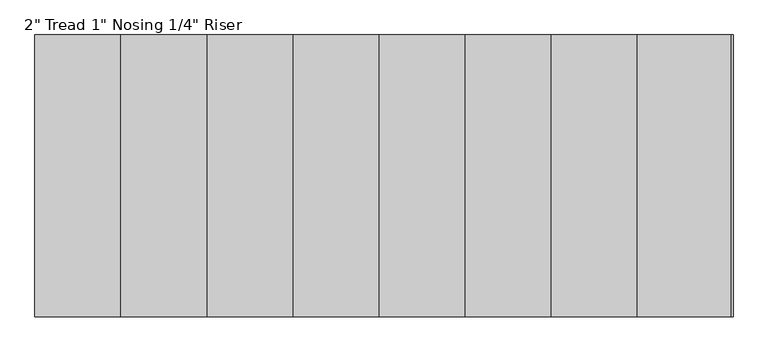
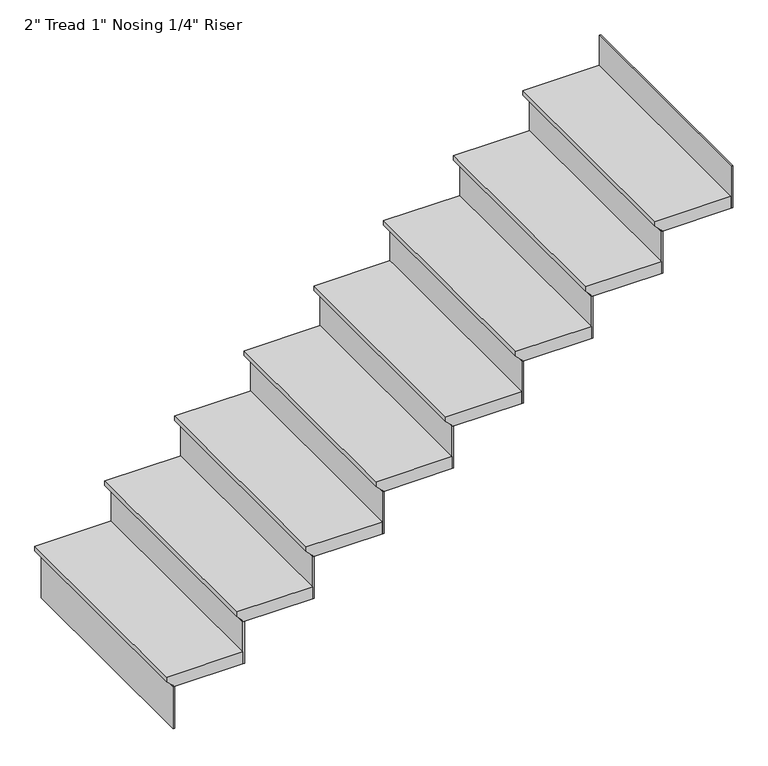
"""IFC4 building model written with IfcOpenShell, lengths in millimetres: stair flight geometry."""

from ifc_helpers import new_model, si_unit, frame, origin, place, context, project, spatial, polyline, outline, extrude, source, transform, mapped, element, save


def stair_flight_0914375a(model_context):
    return source(origin(), model_context, "Body", "SweptSolid", [
        extrude(outline(polyline([(1778.0, -5177.7681702), (1778.0, -5482.5681702), (1758.95, -5482.5681702), (1733.55, -5457.1681702), (1727.2, -5457.1681702), (1727.2, -5177.7681702), (1778.0, -5177.7681702)])), frame((0.0, -6800.457676, 0.0), z_axis=(0.0, 1.0, 0.0), x_axis=(0.0, 0.0, 1.0)), (0.0, 0.0, 1.0), 914.4),
        extrude(outline(polyline([(-5450.8181702, -6800.457676), (-5457.1681702, -6800.457676), (-5457.1681702, -5886.057676), (-5450.8181702, -5886.057676), (-5450.8181702, -6800.457676)])), frame((0.0, 0.0, 1549.4), z_axis=(0.0, 0.0, 1.0), x_axis=(1.0, 0.0, 0.0)), (0.0, 0.0, 1.0), 177.8),
        extrude(outline(polyline([(-3215.6181702, -6800.457676), (-3221.9681702, -6800.457676), (-3221.9681702, -5886.057676), (-3215.6181702, -5886.057676), (-3215.6181702, -6800.457676)])), frame((0.0, 0.0, 2971.8), z_axis=(0.0, 0.0, 1.0), x_axis=(1.0, 0.0, 0.0)), (0.0, 0.0, 1.0), 177.8),
        extrude(outline(polyline([(-5171.4181702, -6800.457676), (-5177.7681702, -6800.457676), (-5177.7681702, -5886.057676), (-5171.4181702, -5886.057676), (-5171.4181702, -6800.457676)])), frame((0.0, 0.0, 1727.2), z_axis=(0.0, 0.0, 1.0), x_axis=(1.0, 0.0, 0.0)), (0.0, 0.0, 1.0), 177.8),
        extrude(outline(polyline([(1955.8, -4898.3681702), (1955.8, -5203.1681702), (1936.75, -5203.1681702), (1911.35, -5177.7681702), (1905.0, -5177.7681702), (1905.0, -4898.3681702), (1955.8, -4898.3681702)])), frame((0.0, -6800.457676, 0.0), z_axis=(0.0, 1.0, 0.0), x_axis=(0.0, 0.0, 1.0)), (0.0, 0.0, 1.0), 914.4),
        extrude(outline(polyline([(-4892.0181702, -6800.457676), (-4898.3681702, -6800.457676), (-4898.3681702, -5886.057676), (-4892.0181702, -5886.057676), (-4892.0181702, -6800.457676)])), frame((0.0, 0.0, 1905.0), z_axis=(0.0, 0.0, 1.0), x_axis=(1.0, 0.0, 0.0)), (0.0, 0.0, 1.0), 177.8),
        extrude(outline(polyline([(2133.6, -4618.9681702), (2133.6, -4923.7681702), (2114.55, -4923.7681702), (2089.15, -4898.3681702), (2082.8, -4898.3681702), (2082.8, -4618.9681702), (2133.6, -4618.9681702)])), frame((0.0, -6800.457676, 0.0), z_axis=(0.0, 1.0, 0.0), x_axis=(0.0, 0.0, 1.0)), (0.0, 0.0, 1.0), 914.4),
        extrude(outline(polyline([(-4612.6181702, -6800.457676), (-4618.9681702, -6800.457676), (-4618.9681702, -5886.057676), (-4612.6181702, -5886.057676), (-4612.6181702, -6800.457676)])), frame((0.0, 0.0, 2082.8), z_axis=(0.0, 0.0, 1.0), x_axis=(1.0, 0.0, 0.0)), (0.0, 0.0, 1.0), 177.8),
        extrude(outline(polyline([(2311.4, -4339.5681702), (2311.4, -4644.3681702), (2292.35, -4644.3681702), (2266.95, -4618.9681702), (2260.6, -4618.9681702), (2260.6, -4339.5681702), (2311.4, -4339.5681702)])), frame((0.0, -6800.457676, 0.0), z_axis=(0.0, 1.0, 0.0), x_axis=(0.0, 0.0, 1.0)), (0.0, 0.0, 1.0), 914.4),
        extrude(outline(polyline([(-4333.2181702, -6800.457676), (-4339.5681702, -6800.457676), (-4339.5681702, -5886.057676), (-4333.2181702, -5886.057676), (-4333.2181702, -6800.457676)])), frame((0.0, 0.0, 2260.6), z_axis=(0.0, 0.0, 1.0), x_axis=(1.0, 0.0, 0.0)), (0.0, 0.0, 1.0), 177.8),
        extrude(outline(polyline([(2489.2, -4060.1681702), (2489.2, -4364.9681702), (2470.15, -4364.9681702), (2444.75, -4339.5681702), (2438.4, -4339.5681702), (2438.4, -4060.1681702), (2489.2, -4060.1681702)])), frame((0.0, -6800.457676, 0.0), z_axis=(0.0, 1.0, 0.0), x_axis=(0.0, 0.0, 1.0)), (0.0, 0.0, 1.0), 914.4),
        extrude(outline(polyline([(-4053.8181702, -6800.457676), (-4060.1681702, -6800.457676), (-4060.1681702, -5886.057676), (-4053.8181702, -5886.057676), (-4053.8181702, -6800.457676)])), frame((0.0, 0.0, 2438.4), z_axis=(0.0, 0.0, 1.0), x_axis=(1.0, 0.0, 0.0)), (0.0, 0.0, 1.0), 177.8),
        extrude(outline(polyline([(2667.0, -3780.7681702), (2667.0, -4085.5681702), (2647.95, -4085.5681702), (2622.55, -4060.1681702), (2616.2, -4060.1681702), (2616.2, -3780.7681702), (2667.0, -3780.7681702)])), frame((0.0, -6800.457676, 0.0), z_axis=(0.0, 1.0, 0.0), x_axis=(0.0, 0.0, 1.0)), (0.0, 0.0, 1.0), 914.4),
        extrude(outline(polyline([(-3774.4181702, -6800.457676), (-3780.7681702, -6800.457676), (-3780.7681702, -5886.057676), (-3774.4181702, -5886.057676), (-3774.4181702, -6800.457676)])), frame((0.0, 0.0, 2616.2), z_axis=(0.0, 0.0, 1.0), x_axis=(1.0, 0.0, 0.0)), (0.0, 0.0, 1.0), 177.8),
        extrude(outline(polyline([(2844.8, -3501.3681702), (2844.8, -3806.1681702), (2825.75, -3806.1681702), (2800.35, -3780.7681702), (2794.0, -3780.7681702), (2794.0, -3501.3681702), (2844.8, -3501.3681702)])), frame((0.0, -6800.457676, 0.0), z_axis=(0.0, 1.0, 0.0), x_axis=(0.0, 0.0, 1.0)), (0.0, 0.0, 1.0), 914.4),
        extrude(outline(polyline([(-3495.0181702, -6800.457676), (-3501.3681702, -6800.457676), (-3501.3681702, -5886.057676), (-3495.0181702, -5886.057676), (-3495.0181702, -6800.457676)])), frame((0.0, 0.0, 2794.0), z_axis=(0.0, 0.0, 1.0), x_axis=(1.0, 0.0, 0.0)), (0.0, 0.0, 1.0), 177.8),
        extrude(outline(polyline([(3022.6, -3221.9681702), (3022.6, -3526.7681702), (3003.55, -3526.7681702), (2978.15, -3501.3681702), (2971.8, -3501.3681702), (2971.8, -3221.9681702), (3022.6, -3221.9681702)])), frame((0.0, -6800.457676, 0.0), z_axis=(0.0, 1.0, 0.0), x_axis=(0.0, 0.0, 1.0)), (0.0, 0.0, 1.0), 914.4),
    ])


if __name__ == "__main__":
    model = new_model("IFC4")
    model_context = context("Model", 3, world=origin())
    ifc_project = project(units=[si_unit("LENGTHUNIT", "METRE", prefix="MILLI")], contexts=[model_context])
    site = spatial("IfcSite", under=ifc_project)
    building = spatial("IfcBuilding", under=site)
    placement = place(None, origin())
    stair_flight_shape = stair_flight_0914375a(model_context)
    element("IfcStairFlight", 1, ObjectType="2\" Tread 1\" Nosing 1/4\" Riser", at=placement, inside=building, context=model_context, shape_type="MappedRepresentation", body=[
        mapped(stair_flight_shape, transform((0.0, 0.0, 0.0), x_axis=(1.0, 0.0, 0.0), y_axis=(0.0, 1.0, 0.0), z_axis=(0.0, 0.0, 1.0))),
    ])
    save(model, "model.ifc")
